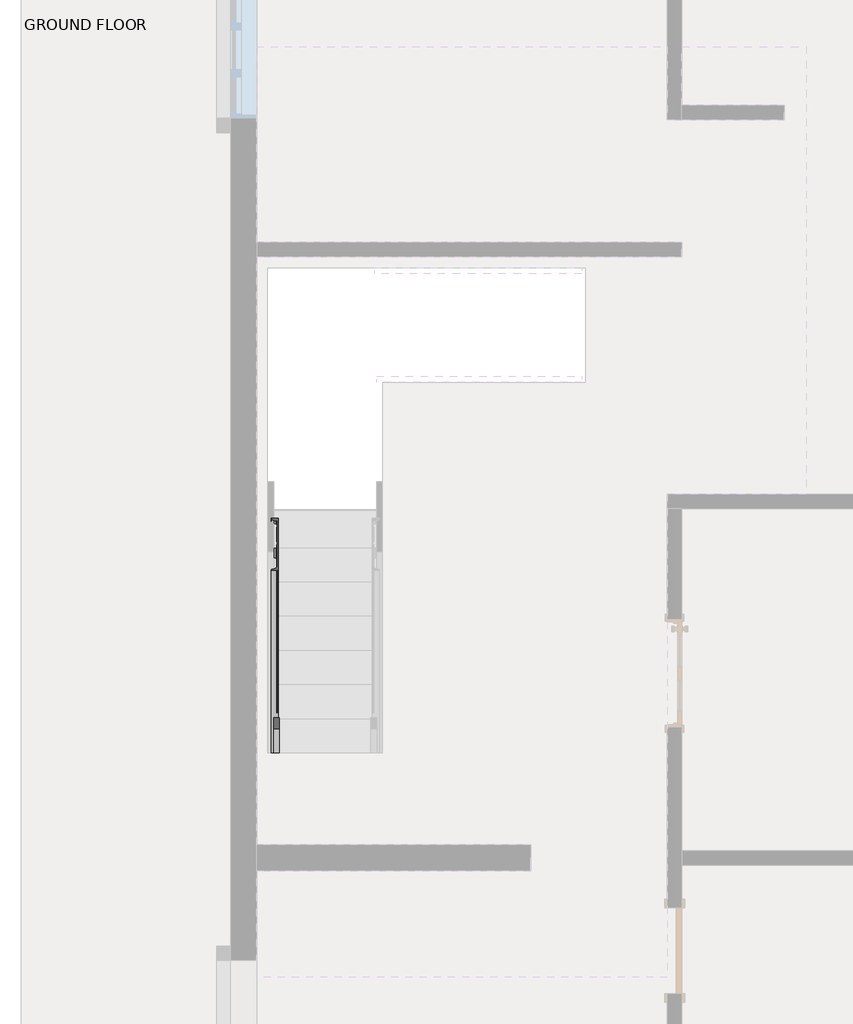
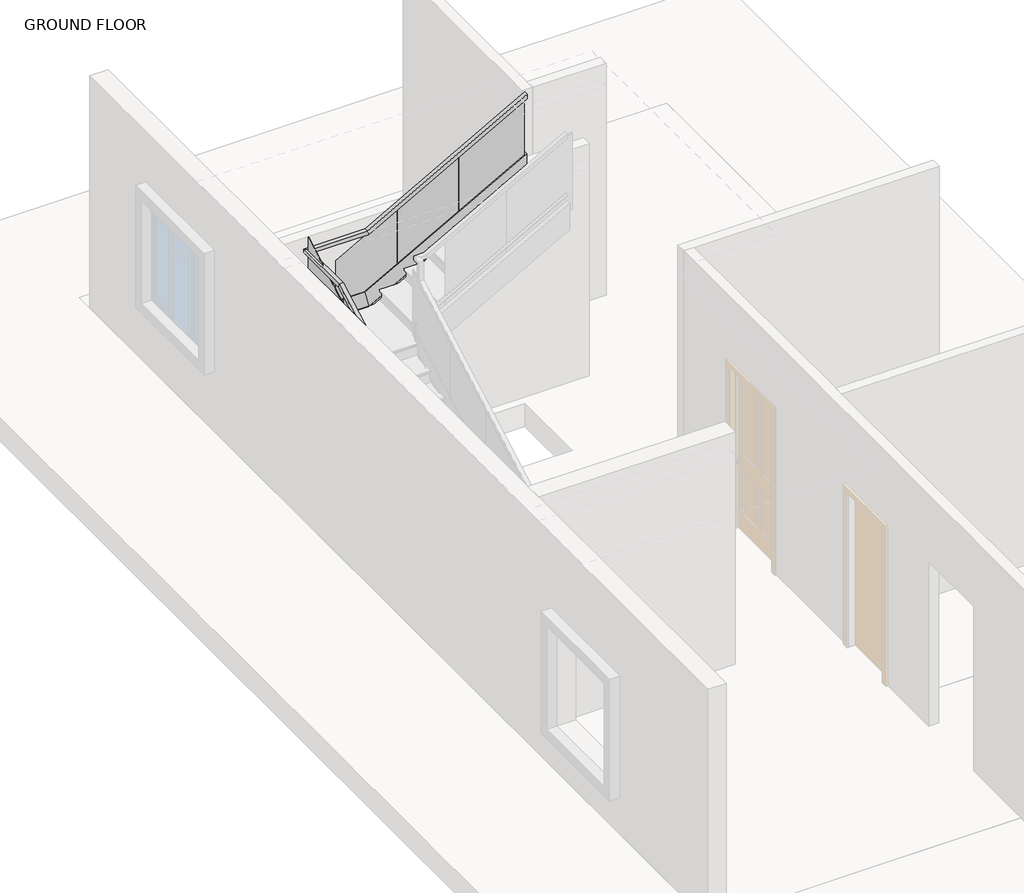
# One storey, part 3 of 4: 1 railing.
"""IFC4 building model written with IfcOpenShell, lengths in millimetres."""

from ifc_helpers import new_model, si_unit, frame, origin, place, context, project, spatial, polyline, circle_curve, ellipse_curve, outline, extrude, faceted_brep, element, save
from ifc_brep_helpers import plane_surface, cylinder_surface, revolved_surface, advanced_brep

model = new_model("IFC4")

# Units and contexts
model_context = context("Model", 3, world=origin())
ifc_project = project(units=[si_unit("LENGTHUNIT", "METRE", prefix="MILLI")], contexts=[model_context])

# Site, building, storey
site = spatial("IfcSite", under=ifc_project)
building = spatial("IfcBuilding", under=site)
storey = spatial("IfcBuildingStorey", under=building, Name="GROUND FLOOR", Elevation=304.8)

# Railing
placement = place(None, origin())
element("IfcRailing", 1, ObjectType="GLASS PANEL RAILING", at=placement, inside=storey, context=model_context, shape_type="SolidModel", body=[
    faceted_brep([(-9317.1482439, -642.5827462, 1388.5333333), (-9317.1482439, -642.5827462, 1330.420221), (-9266.3482439, -642.5827462, 1330.420221), (-9266.3482439, -642.5827462, 1388.5333333), (-9317.1482439, 2861.8235038, 3335.4256944), (-9317.1482439, 2874.9871061, 3284.6256944), (-9266.3482439, 2874.9871061, 3284.6256944), (-9266.3482439, 2861.8235038, 3335.4256944), (-9317.1482439, 3624.6172538, 3335.4256944), (-9317.1482439, 3624.6172538, 3284.6256944), (-9266.3482439, 3573.8172538, 3284.6256944), (-9266.3482439, 3573.8172538, 3335.4256944), (-8554.3544939, 3624.6172538, 3335.4256944), (-8541.1908917, 3624.6172538, 3284.6256944), (-8541.1908917, 3573.8172538, 3284.6256944), (-8554.3544939, 3573.8172538, 3335.4256944), (-6572.3607439, 3624.6172538, 4436.5333333), (-6572.3607439, 3573.8172538, 4436.5333333), (-6572.3607439, 3573.8172538, 4378.420221), (-6572.3607439, 3624.6172538, 4378.420221)], [[[0, 1, 2, 3]], [[1, 0, 4, 5]], [[2, 1, 5, 6]], [[3, 2, 6, 7]], [[0, 3, 7, 4]], [[5, 4, 8, 9]], [[6, 5, 9, 10]], [[7, 6, 10, 11]], [[4, 7, 11, 8]], [[9, 8, 12, 13]], [[10, 9, 13, 14]], [[11, 10, 14, 15]], [[8, 11, 15, 12]], [[16, 17, 18, 19]], [[13, 12, 16, 19]], [[14, 13, 19, 18]], [[15, 14, 18, 17]], [[12, 15, 17, 16]]]),
    advanced_brep(
    [(-9276.8638439, -642.5827462, 604.8878361), (-9340.1098439, -642.5827462, 604.8878361), (-9340.1098439, -642.5827462, 603.3095437), (-9335.7270347, -642.5827462, 597.391004), (-9312.1063439, -642.5827462, 592.8874784), (-9292.8684623, -642.5827462, 589.2195801), (-9284.1028439, -642.5827462, 577.3825008), (-9284.1028439, -642.5827462, 370.8841659), (-9292.8684623, -642.5827462, 359.0470866), (-9312.1063439, -642.5827462, 355.3791882), (-9335.7270347, -642.5827462, 350.8756626), (-9340.1098439, -642.5827462, 344.957123), (-9340.1098439, -642.5827462, 343.3788305), (-9276.8638439, -642.5827462, 343.3788305), (-9276.8638439, 2832.2053988, 2535.3256944), (-9340.1098439, 2832.2053988, 2535.3256944), (-9340.1098439, 2832.5629087, 2533.9460186), (-9335.7270347, 2833.903558, 2528.7722841), (-9312.1063439, 2834.9236827, 2524.8354944), (-9292.8684623, 2835.7545237, 2521.6291744), (-9284.1028439, 2838.4358222, 2511.2817054), (-9284.1028439, 2885.2111855, 2330.7696834), (-9292.8684623, 2887.892484, 2320.4222145), (-9312.1063439, 2888.723325, 2317.2158944), (-9335.7270347, 2889.7434497, 2313.2791048), (-9340.1098439, 2891.0840989, 2308.1053703), (-9340.1098439, 2891.4416089, 2306.7256944), (-9276.8638439, 2891.4416089, 2306.7256944), (-9276.8638439, 3584.3328538, 2535.3256944), (-9276.8638439, 3584.3328538, 2306.7256944), (-9340.1098439, 3584.3328538, 2306.7256944), (-9340.1098439, 3584.3328538, 2308.1053703), (-9335.7270347, 3584.3328538, 2313.2791048), (-9312.1063439, 3584.3328538, 2317.2158944), (-9292.8684623, 3584.3328538, 2320.4222145), (-9284.1028439, 3584.3328538, 2330.7696834), (-9284.1028439, 3584.3328538, 2511.2817054), (-9292.8684623, 3584.3328538, 2521.6291744), (-9312.1063439, 3584.3328538, 2524.8354944), (-9335.7270347, 3584.3328538, 2528.7722841), (-9340.1098439, 3584.3328538, 2533.9460186), (-9340.1098439, 3584.3328538, 2535.3256944)],
    [
        (0, 1),
        (1, 2),
        (2, 3, ellipse_curve(frame((-9334.8647439, -642.5827462, 603.3095437), z_axis=(0.0, -1.0, 0.0), x_axis=(0.0, 0.0, -1.0)), 6.0001789, 5.2451)),
        (3, 4),
        (4, 5),
        (5, 6, ellipse_curve(frame((-9294.5930439, -642.5827462, 577.3825008), z_axis=(0.0, 1.0, 0.0), x_axis=(0.0, 0.0, 1.0)), 12.0003577, 10.4902)),
        (6, 7),
        (7, 8, ellipse_curve(frame((-9294.5930439, -642.5827462, 370.8841659), z_axis=(0.0, 1.0, 0.0), x_axis=(0.0, 0.0, 1.0)), 12.0003577, 10.4902)),
        (8, 9),
        (9, 10),
        (10, 11, ellipse_curve(frame((-9334.8647439, -642.5827462, 344.957123), z_axis=(0.0, -1.0, 0.0), x_axis=(0.0, 0.0, -1.0)), 6.0001789, 5.2451)),
        (11, 12),
        (12, 13),
        (13, 0),
        (0, 14),
        (14, 15),
        (15, 1),
        (15, 16),
        (16, 2),
        (16, 17, ellipse_curve(frame((-9334.8647439, 2832.5629087, 2533.9460186), z_axis=(0.0, -0.9680282217274294, -0.25084130827922024), x_axis=(0.0, 0.25084130827922074, -0.9680282217274293)), 5.4183338, 5.2451)),
        (17, 3),
        (17, 18),
        (18, 4),
        (18, 19),
        (19, 5),
        (19, 20, ellipse_curve(frame((-9294.5930439, 2838.4358222, 2511.2817054), z_axis=(0.0, 0.9680282217274294, 0.25084130827922024), x_axis=(0.0, -0.25084130827922074, 0.9680282217274293)), 10.8366675, 10.4902)),
        (20, 6),
        (20, 21),
        (21, 7),
        (21, 22, ellipse_curve(frame((-9294.5930439, 2885.2111855, 2330.7696834), z_axis=(0.0, 0.9680282217274294, 0.25084130827922024), x_axis=(0.0, -0.25084130827922074, 0.9680282217274293)), 10.8366675, 10.4902)),
        (22, 8),
        (22, 23),
        (23, 9),
        (23, 24),
        (24, 10),
        (24, 25, ellipse_curve(frame((-9334.8647439, 2891.0840989, 2308.1053703), z_axis=(0.0, -0.9680282217274294, -0.25084130827922024), x_axis=(0.0, 0.25084130827922074, -0.9680282217274293)), 5.4183338, 5.2451)),
        (25, 11),
        (25, 26),
        (26, 12),
        (26, 27),
        (27, 13),
        (27, 14),
        (28, 29),
        (29, 30),
        (30, 31),
        (31, 32, circle_curve(frame((-9334.8647439, 3584.3328538, 2308.1053703), z_axis=(0.0, 1.0, 0.0), x_axis=(-1.0, 0.0, 0.0)), 5.2451)),
        (32, 33),
        (33, 34),
        (34, 35, circle_curve(frame((-9294.5930439, 3584.3328538, 2330.7696834), z_axis=(0.0, -1.0, 0.0), x_axis=(-1.0, 0.0, 0.0)), 10.4902)),
        (35, 36),
        (36, 37, circle_curve(frame((-9294.5930439, 3584.3328538, 2511.2817054), z_axis=(0.0, -1.0, 0.0), x_axis=(-1.0, 0.0, 0.0)), 10.4902)),
        (37, 38),
        (38, 39),
        (39, 40, circle_curve(frame((-9334.8647439, 3584.3328538, 2533.9460186), z_axis=(0.0, 1.0, 0.0), x_axis=(-1.0, 0.0, 0.0)), 5.2451)),
        (40, 41),
        (41, 28),
        (14, 28),
        (41, 15),
        (40, 16),
        (39, 17),
        (38, 18),
        (37, 19),
        (36, 20),
        (35, 21),
        (34, 22),
        (33, 23),
        (32, 24),
        (31, 25),
        (30, 26),
        (29, 27),
    ],
    [
        plane_surface(frame((-9291.7482439, -642.5827462, 474.1333333), z_axis=(0.0, -1.0, 0.0), x_axis=(0.0, 0.0, 1.0))),
        plane_surface(frame((-9276.8638439, -642.5827462, 604.8878361), z_axis=(0.0, -0.48564293117863094, 0.8741572761215385), x_axis=(0.0, 0.8741572761215385, 0.48564293117863094))),
        plane_surface(frame((-9340.1098439, -642.5827462, 604.8878361), z_axis=(-1.0, 0.0, 0.0), x_axis=(0.0, 0.8741572761215384, 0.4856429311786311))),
        cylinder_surface(frame((-9334.8647439, -697.4217034, 572.8434563), z_axis=(0.0, -0.8741572761215384, -0.48564293117863094), x_axis=(-1.0, 0.0, 0.0)), 5.2451),
        plane_surface(frame((-9335.7270347, -642.5827462, 597.391004), z_axis=(-0.16439930721687, 0.47903521057281384, -0.862263379031067), x_axis=(0.0, 0.8741572761215385, 0.48564293117863105))),
        plane_surface(frame((-9312.1063439, -642.5827462, 592.8874784), z_axis=(-0.16439930721687057, 0.4790352105728138, -0.8622633790310668), x_axis=(0.0, 0.8741572761215384, 0.48564293117863105))),
        revolved_surface(polyline([(-9305.0832439, 2840.8120297710066, 2512.6018208061087), (-9305.0832439, -647.677237685849, 574.5522277745283)]), (-9294.5930439, -686.4149399, 553.0312821), (0.0, 0.8741572761215384, 0.48564293117863094)),
        plane_surface(frame((-9284.1028439, -642.5827462, 577.3825008), z_axis=(-1.0, 0.0, 0.0), x_axis=(0.0, 0.8741572761215384, 0.485642931178631))),
        revolved_surface(polyline([(-9305.0832439, 2887.587393094591, 2332.0897987636554), (-9305.0832439, -647.6772376433962, 368.0538927981132)]), (-9294.5930439, -598.7505524, 395.2353846), (0.0, 0.8741572761215384, 0.48564293117863094)),
        plane_surface(frame((-9292.8684623, -642.5827462, 359.0470866), z_axis=(-0.16439930721687776, -0.4790352105728128, 0.862263379031066), x_axis=(0.0, 0.8741572761215384, 0.485642931178631))),
        plane_surface(frame((-9312.1063439, -642.5827462, 355.3791882), z_axis=(-0.1643993072168788, -0.4790352105728126, 0.8622633790310659), x_axis=(0.0, 0.8741572761215384, 0.48564293117863094))),
        cylinder_surface(frame((-9334.8647439, -587.7437889, 375.4232103), z_axis=(0.0, -0.8741572761215384, -0.48564293117863094), x_axis=(-1.0, 0.0, 0.0)), 5.2451),
        plane_surface(frame((-9340.1098439, -642.5827462, 344.957123), z_axis=(-1.0, 0.0, 0.0), x_axis=(0.0, 0.8741572761215384, 0.485642931178631))),
        plane_surface(frame((-9340.1098439, -642.5827462, 343.3788305), z_axis=(0.0, 0.48564293117863094, -0.8741572761215385), x_axis=(0.0, 0.8741572761215385, 0.48564293117863094))),
        plane_surface(frame((-9276.8638439, -642.5827462, 343.3788305), z_axis=(1.0000000000000002, 0.0, 0.0), x_axis=(0.0, 0.8741572761215385, 0.48564293117863094))),
        plane_surface(frame((-9291.7482439, 3584.3328538, 2421.0256944), z_axis=(0.0, 1.0, 0.0), x_axis=(0.0, 0.0, 1.0))),
        plane_surface(frame((-9276.8638439, 2832.2053988, 2535.3256944), z_axis=(0.0, 0.0, 1.0), x_axis=(0.0, 1.0, 0.0))),
        plane_surface(frame((-9340.1098439, 2832.2053988, 2535.3256944), z_axis=(-1.0, 0.0, 0.0), x_axis=(0.0, 1.0, 0.0))),
        cylinder_surface(frame((-9334.8647439, 2861.8235038, 2533.9460186), z_axis=(0.0, -1.0, 0.0), x_axis=(-1.0, 0.0, 0.0)), 5.2451),
        plane_surface(frame((-9335.7270347, 2833.903558, 2528.7722841), z_axis=(-0.16439930721687074, 0.0, -0.9863938705135049), x_axis=(0.0, 1.0, 0.0))),
        plane_surface(frame((-9312.1063439, 2834.9236827, 2524.8354944), z_axis=(-0.16439930721687138, 0.0, -0.9863938705135048), x_axis=(0.0, 1.0, 0.0))),
        revolved_surface(polyline([(-9305.0832439, 3584.3328538, 2511.2817054), (-9305.0832439, 2835.717538346913, 2511.2817054)]), (-9294.5930439, 2861.8235038, 2511.2817054), (0.0, 1.0, 0.0)),
        plane_surface(frame((-9284.1028439, 2838.4358222, 2511.2817054), z_axis=(-1.0, 0.0, 0.0), x_axis=(0.0, 1.0, 0.0))),
        revolved_surface(polyline([(-9305.0832439, 3584.3328538, 2330.7696834), (-9305.0832439, 2882.4929016469127, 2330.7696834)]), (-9294.5930439, 2861.8235038, 2330.7696834), (0.0, 1.0, 0.0)),
        plane_surface(frame((-9292.8684623, 2887.892484, 2320.4222145), z_axis=(-0.16439930721687698, 0.0, 0.9863938705135039), x_axis=(0.0, 1.0, 0.0))),
        plane_surface(frame((-9312.1063439, 2888.723325, 2317.2158944), z_axis=(-0.164399307216878, 0.0, 0.9863938705135037), x_axis=(0.0, 1.0, 0.0))),
        cylinder_surface(frame((-9334.8647439, 2861.8235038, 2308.1053703), z_axis=(0.0, -1.0, 0.0), x_axis=(-1.0, 0.0, 0.0)), 5.2451),
        plane_surface(frame((-9340.1098439, 2891.0840989, 2308.1053703), z_axis=(-1.0, 0.0, 0.0), x_axis=(0.0, 1.0, 0.0))),
        plane_surface(frame((-9340.1098439, 2891.4416089, 2306.7256944), z_axis=(0.0, 0.0, -1.0), x_axis=(0.0, 1.0, 0.0))),
        plane_surface(frame((-9276.8638439, 2891.4416089, 2306.7256944), z_axis=(1.0, 0.0, 0.0), x_axis=(0.0, 1.0, 0.0))),
    ],
    [
        (0, [[1, 2, 3, 4, 5, 6, 7, 8, 9, 10, 11, 12, 13, 14]]),
        (1, [[-1, 15, 16, 17]]),
        (2, [[-2, -17, 18, 19]]),
        (3, [[-3, -19, 20, 21]]),
        (4, [[-4, -21, 22, 23]]),
        (5, [[-5, -23, 24, 25]]),
        (6, [[-6, -25, 26, 27]]),
        (7, [[-7, -27, 28, 29]]),
        (8, [[-8, -29, 30, 31]]),
        (9, [[-9, -31, 32, 33]]),
        (10, [[-10, -33, 34, 35]]),
        (11, [[-11, -35, 36, 37]]),
        (12, [[-12, -37, 38, 39]]),
        (13, [[-13, -39, 40, 41]]),
        (14, [[-14, -41, 42, -15]]),
        (15, [[43, 44, 45, 46, 47, 48, 49, 50, 51, 52, 53, 54, 55, 56]]),
        (16, [[-16, 57, -56, 58]]),
        (17, [[-18, -58, -55, 59]]),
        (18, [[-20, -59, -54, 60]]),
        (19, [[-22, -60, -53, 61]]),
        (20, [[-24, -61, -52, 62]]),
        (21, [[-26, -62, -51, 63]]),
        (22, [[-28, -63, -50, 64]]),
        (23, [[-30, -64, -49, 65]]),
        (24, [[-32, -65, -48, 66]]),
        (25, [[-34, -66, -47, 67]]),
        (26, [[-36, -67, -46, 68]]),
        (27, [[-38, -68, -45, 69]]),
        (28, [[-40, -69, -44, 70]]),
        (29, [[-42, -70, -43, -57]]),
    ],
),
    advanced_brep(
    [(-9340.1098439, 3584.3328538, 2535.3256944), (-9340.1098439, 3647.5788538, 2535.3256944), (-9340.1098439, 3647.5788538, 2533.9460186), (-9340.1098439, 3643.1960447, 2528.7722841), (-9340.1098439, 3619.5753538, 2524.8354944), (-9340.1098439, 3600.3374722, 2521.6291744), (-9340.1098439, 3591.5718538, 2511.2817054), (-9340.1098439, 3591.5718538, 2330.7696834), (-9340.1098439, 3600.3374722, 2320.4222145), (-9340.1098439, 3619.5753538, 2317.2158944), (-9340.1098439, 3643.1960447, 2313.2791048), (-9340.1098439, 3647.5788538, 2308.1053703), (-9340.1098439, 3647.5788538, 2306.7256944), (-9340.1098439, 3584.3328538, 2306.7256944), (-8583.9725989, 3584.3328538, 2535.3256944), (-8583.9725989, 3647.5788538, 2535.3256944), (-8583.615089, 3647.5788538, 2533.9460186), (-8582.2744397, 3643.1960447, 2528.7722841), (-8581.2543151, 3619.5753538, 2524.8354944), (-8580.4234741, 3600.3374722, 2521.6291744), (-8577.7421756, 3591.5718538, 2511.2817054), (-8530.9668123, 3591.5718538, 2330.7696834), (-8528.2855137, 3600.3374722, 2320.4222145), (-8527.4546728, 3619.5753538, 2317.2158944), (-8526.4345481, 3643.1960447, 2313.2791048), (-8525.0938988, 3647.5788538, 2308.1053703), (-8524.7363889, 3647.5788538, 2306.7256944), (-8524.7363889, 3584.3328538, 2306.7256944), (-6572.3607439, 3584.3328538, 3652.8878361), (-6572.3607439, 3584.3328538, 3391.3788305), (-6572.3607439, 3647.5788538, 3391.3788305), (-6572.3607439, 3647.5788538, 3392.957123), (-6572.3607439, 3643.1960447, 3398.8756626), (-6572.3607439, 3619.5753538, 3403.3791882), (-6572.3607439, 3600.3374722, 3407.0470866), (-6572.3607439, 3591.5718538, 3418.8841659), (-6572.3607439, 3591.5718538, 3625.3825008), (-6572.3607439, 3600.3374722, 3637.2195801), (-6572.3607439, 3619.5753538, 3640.8874784), (-6572.3607439, 3643.1960447, 3645.391004), (-6572.3607439, 3647.5788538, 3651.3095437), (-6572.3607439, 3647.5788538, 3652.8878361)],
    [
        (0, 1),
        (1, 2),
        (2, 3, circle_curve(frame((-9340.1098439, 3642.3337538, 2533.9460186), z_axis=(-1.0, 0.0, 0.0), x_axis=(0.0, 1.0, 0.0)), 5.2451)),
        (3, 4),
        (4, 5),
        (5, 6, circle_curve(frame((-9340.1098439, 3602.0620538, 2511.2817054), z_axis=(1.0, 0.0, 0.0), x_axis=(0.0, 1.0, 0.0)), 10.4902)),
        (6, 7),
        (7, 8, circle_curve(frame((-9340.1098439, 3602.0620538, 2330.7696834), z_axis=(1.0, 0.0, 0.0), x_axis=(0.0, 1.0, 0.0)), 10.4902)),
        (8, 9),
        (9, 10),
        (10, 11, circle_curve(frame((-9340.1098439, 3642.3337538, 2308.1053703), z_axis=(-1.0, 0.0, 0.0), x_axis=(0.0, 1.0, 0.0)), 5.2451)),
        (11, 12),
        (12, 13),
        (13, 0),
        (0, 14),
        (14, 15),
        (15, 1),
        (15, 16),
        (16, 2),
        (16, 17, ellipse_curve(frame((-8583.615089, 3642.3337538, 2533.9460186), z_axis=(-0.9680282217274294, 0.0, -0.2508413082792203), x_axis=(-0.2508413082792198, 0.0, 0.9680282217274295)), 5.4183338, 5.2451)),
        (17, 3),
        (17, 18),
        (18, 4),
        (18, 19),
        (19, 5),
        (19, 20, ellipse_curve(frame((-8577.7421756, 3602.0620538, 2511.2817054), z_axis=(0.9680282217274294, 0.0, 0.2508413082792203), x_axis=(0.2508413082792198, 0.0, -0.9680282217274295)), 10.8366675, 10.4902)),
        (20, 6),
        (20, 21),
        (21, 7),
        (21, 22, ellipse_curve(frame((-8530.9668123, 3602.0620538, 2330.7696834), z_axis=(0.9680282217274294, 0.0, 0.2508413082792203), x_axis=(0.2508413082792198, 0.0, -0.9680282217274295)), 10.8366675, 10.4902)),
        (22, 8),
        (22, 23),
        (23, 9),
        (23, 24),
        (24, 10),
        (24, 25, ellipse_curve(frame((-8525.0938988, 3642.3337538, 2308.1053703), z_axis=(-0.9680282217274294, 0.0, -0.2508413082792203), x_axis=(-0.2508413082792198, 0.0, 0.9680282217274295)), 5.4183338, 5.2451)),
        (25, 11),
        (25, 26),
        (26, 12),
        (26, 27),
        (27, 13),
        (27, 14),
        (28, 29),
        (29, 30),
        (30, 31),
        (31, 32, ellipse_curve(frame((-6572.3607439, 3642.3337538, 3392.957123), z_axis=(1.0, 0.0, 0.0), x_axis=(0.0, 0.0, -1.0)), 6.0001789, 5.2451)),
        (32, 33),
        (33, 34),
        (34, 35, ellipse_curve(frame((-6572.3607439, 3602.0620538, 3418.8841659), z_axis=(-1.0, 0.0, 0.0), x_axis=(0.0, 0.0, 1.0)), 12.0003577, 10.4902)),
        (35, 36),
        (36, 37, ellipse_curve(frame((-6572.3607439, 3602.0620538, 3625.3825008), z_axis=(-1.0, 0.0, 0.0), x_axis=(0.0, 0.0, 1.0)), 12.0003577, 10.4902)),
        (37, 38),
        (38, 39),
        (39, 40, ellipse_curve(frame((-6572.3607439, 3642.3337538, 3651.3095437), z_axis=(1.0, 0.0, 0.0), x_axis=(0.0, 0.0, -1.0)), 6.0001789, 5.2451)),
        (40, 41),
        (41, 28),
        (14, 28),
        (41, 15),
        (40, 16),
        (39, 17),
        (38, 18),
        (37, 19),
        (36, 20),
        (35, 21),
        (34, 22),
        (33, 23),
        (32, 24),
        (31, 25),
        (30, 26),
        (29, 27),
    ],
    [
        plane_surface(frame((-9340.1098439, 3599.2172538, 2421.0256944), z_axis=(-1.0, 0.0, 0.0), x_axis=(0.0, 1.0, 0.0))),
        plane_surface(frame((-9340.1098439, 3584.3328538, 2535.3256944), z_axis=(0.0, 0.0, 1.0), x_axis=(1.0, 0.0, 0.0))),
        plane_surface(frame((-9340.1098439, 3647.5788538, 2535.3256944), z_axis=(0.0, 1.0, 0.0), x_axis=(1.0, 0.0, 0.0))),
        cylinder_surface(frame((-9340.1098439, 3642.3337538, 2533.9460186), z_axis=(-1.0, 0.0, 0.0), x_axis=(0.0, 1.0, 0.0)), 5.2451),
        plane_surface(frame((-9340.1098439, 3643.1960447, 2528.7722841), z_axis=(0.0, 0.16439930721687082, -0.9863938705135049), x_axis=(1.0, 0.0, 0.0))),
        plane_surface(frame((-9340.1098439, 3619.5753538, 2524.8354944), z_axis=(0.0, 0.16439930721687146, -0.9863938705135048), x_axis=(1.0, 0.0, 0.0))),
        revolved_surface(polyline([(-8575.023891746914, 3612.5522538, 2511.2817054), (-9340.1098439, 3612.5522538, 2511.2817054)]), (-9340.1098439, 3602.0620538, 2511.2817054), (1.0, 0.0, 0.0)),
        plane_surface(frame((-9340.1098439, 3591.5718538, 2511.2817054), z_axis=(0.0, 1.0, 0.0), x_axis=(1.0, 0.0, 0.0))),
        revolved_surface(polyline([(-8528.248528446913, 3612.5522538, 2330.7696834), (-9340.1098439, 3612.5522538, 2330.7696834)]), (-9340.1098439, 3602.0620538, 2330.7696834), (1.0, 0.0, 0.0)),
        plane_surface(frame((-9340.1098439, 3600.3374722, 2320.4222145), z_axis=(0.0, 0.1643993072168769, 0.9863938705135039), x_axis=(1.0, 0.0, 0.0))),
        plane_surface(frame((-9340.1098439, 3619.5753538, 2317.2158944), z_axis=(0.0, 0.16439930721687793, 0.9863938705135037), x_axis=(1.0, 0.0, 0.0))),
        cylinder_surface(frame((-9340.1098439, 3642.3337538, 2308.1053703), z_axis=(-1.0, 0.0, 0.0), x_axis=(0.0, 1.0, 0.0)), 5.2451),
        plane_surface(frame((-9340.1098439, 3647.5788538, 2308.1053703), z_axis=(0.0, 1.0, 0.0), x_axis=(1.0, 0.0, 0.0))),
        plane_surface(frame((-9340.1098439, 3647.5788538, 2306.7256944), z_axis=(0.0, 0.0, -1.0), x_axis=(1.0, 0.0, 0.0))),
        plane_surface(frame((-9340.1098439, 3584.3328538, 2306.7256944), z_axis=(0.0, -1.0, 0.0), x_axis=(1.0, 0.0, 0.0))),
        plane_surface(frame((-6572.3607439, 3599.2172538, 3522.1333333), z_axis=(1.0, 0.0, 0.0), x_axis=(0.0, 1.0, 0.0))),
        plane_surface(frame((-8583.9725989, 3584.3328538, 2535.3256944), z_axis=(-0.4856429311786311, 0.0, 0.8741572761215384), x_axis=(0.8741572761215384, 0.0, 0.4856429311786311))),
        plane_surface(frame((-8583.9725989, 3647.5788538, 2535.3256944), z_axis=(0.0, 1.0, 0.0), x_axis=(0.8741572761215384, 0.0, 0.4856429311786311))),
        cylinder_surface(frame((-8609.1934511, 3642.3337538, 2519.7358174), z_axis=(-0.8741572761215384, 0.0, -0.48564293117863105), x_axis=(0.0, 1.0, 0.0)), 5.2451),
        plane_surface(frame((-8582.2744397, 3643.1960447, 2528.7722841), z_axis=(0.47903521057281395, 0.1643993072168694, -0.862263379031067), x_axis=(0.8741572761215385, 0.0, 0.48564293117863094))),
        plane_surface(frame((-8581.2543151, 3619.5753538, 2524.8354944), z_axis=(0.47903521057281423, 0.16439930721687004, -0.8622633790310666), x_axis=(0.8741572761215383, 0.0, 0.4856429311786313))),
        revolved_surface(polyline([(-6567.2662524518855, 3612.5522538, 3628.212773893393), (-8580.11838324176, 3612.5522538, 2509.9615901212446)]), (-8598.1866877, 3602.0620538, 2499.9236432), (0.8741572761215384, 0.0, 0.48564293117863105)),
        plane_surface(frame((-8577.7421756, 3591.5718538, 2511.2817054), z_axis=(0.0, 1.0000000000000002, 0.0), x_axis=(0.8741572761215385, 0.0, 0.48564293117863094))),
        revolved_surface(polyline([(-6567.266252409432, 3612.5522538, 3421.714438916979), (-8533.343019918173, 3612.5522538, 2329.449568078793)]), (-8510.5223002, 3602.0620538, 2342.1277457), (0.8741572761215384, 0.0, 0.48564293117863105)),
        plane_surface(frame((-8528.2855137, 3600.3374722, 2320.4222145), z_axis=(-0.4790352105728125, 0.16439930721687834, 0.8622633790310661), x_axis=(0.8741572761215384, 0.0, 0.48564293117863094))),
        plane_surface(frame((-8527.4546728, 3619.5753538, 2317.2158944), z_axis=(-0.4790352105728125, 0.16439930721687937, 0.8622633790310658), x_axis=(0.8741572761215384, 0.0, 0.4856429311786311))),
        cylinder_surface(frame((-8499.5155367, 3642.3337538, 2322.3155715), z_axis=(-0.8741572761215384, 0.0, -0.48564293117863105), x_axis=(0.0, 1.0, 0.0)), 5.2451),
        plane_surface(frame((-8525.0938988, 3647.5788538, 2308.1053703), z_axis=(0.0, 1.0, 0.0), x_axis=(0.8741572761215384, 0.0, 0.4856429311786311))),
        plane_surface(frame((-8524.7363889, 3647.5788538, 2306.7256944), z_axis=(0.4856429311786312, 0.0, -0.8741572761215383), x_axis=(0.8741572761215383, 0.0, 0.4856429311786312))),
        plane_surface(frame((-8524.7363889, 3584.3328538, 2306.7256944), z_axis=(0.0, -1.0000000000000002, 0.0), x_axis=(0.8741572761215384, 0.0, 0.48564293117863117))),
    ],
    [
        (0, [[1, 2, 3, 4, 5, 6, 7, 8, 9, 10, 11, 12, 13, 14]]),
        (1, [[-1, 15, 16, 17]]),
        (2, [[-2, -17, 18, 19]]),
        (3, [[-3, -19, 20, 21]]),
        (4, [[-4, -21, 22, 23]]),
        (5, [[-5, -23, 24, 25]]),
        (6, [[-6, -25, 26, 27]]),
        (7, [[-7, -27, 28, 29]]),
        (8, [[-8, -29, 30, 31]]),
        (9, [[-9, -31, 32, 33]]),
        (10, [[-10, -33, 34, 35]]),
        (11, [[-11, -35, 36, 37]]),
        (12, [[-12, -37, 38, 39]]),
        (13, [[-13, -39, 40, 41]]),
        (14, [[-14, -41, 42, -15]]),
        (15, [[43, 44, 45, 46, 47, 48, 49, 50, 51, 52, 53, 54, 55, 56]]),
        (16, [[-16, 57, -56, 58]]),
        (17, [[-18, -58, -55, 59]]),
        (18, [[-20, -59, -54, 60]]),
        (19, [[-22, -60, -53, 61]]),
        (20, [[-24, -61, -52, 62]]),
        (21, [[-26, -62, -51, 63]]),
        (22, [[-28, -63, -50, 64]]),
        (23, [[-30, -64, -49, 65]]),
        (24, [[-32, -65, -48, 66]]),
        (25, [[-34, -66, -47, 67]]),
        (26, [[-36, -67, -46, 68]]),
        (27, [[-38, -68, -45, 69]]),
        (28, [[-40, -69, -44, 70]]),
        (29, [[-42, -70, -43, -57]]),
    ],
),
    advanced_brep(
    [(-9276.8638439, -642.5827462, 604.8878361), (-9340.1098439, -642.5827462, 604.8878361), (-9340.1098439, -642.5827462, 603.3095437), (-9335.7270347, -642.5827462, 597.391004), (-9312.1063439, -642.5827462, 592.8874784), (-9292.8684623, -642.5827462, 589.2195801), (-9284.1028439, -642.5827462, 577.3825008), (-9284.1028439, -642.5827462, 370.8841659), (-9292.8684623, -642.5827462, 359.0470866), (-9312.1063439, -642.5827462, 355.3791882), (-9335.7270347, -642.5827462, 350.8756626), (-9340.1098439, -642.5827462, 344.957123), (-9340.1098439, -642.5827462, 343.3788305), (-9276.8638439, -642.5827462, 343.3788305), (-9276.8638439, 2832.2053988, 2535.3256944), (-9340.1098439, 2832.2053988, 2535.3256944), (-9340.1098439, 2832.5629087, 2533.9460186), (-9335.7270347, 2833.903558, 2528.7722841), (-9312.1063439, 2834.9236827, 2524.8354944), (-9292.8684623, 2835.7545237, 2521.6291744), (-9284.1028439, 2838.4358222, 2511.2817054), (-9284.1028439, 2885.2111855, 2330.7696834), (-9292.8684623, 2887.892484, 2320.4222145), (-9312.1063439, 2888.723325, 2317.2158944), (-9335.7270347, 2889.7434497, 2313.2791048), (-9340.1098439, 2891.0840989, 2308.1053703), (-9340.1098439, 2891.4416089, 2306.7256944), (-9276.8638439, 2891.4416089, 2306.7256944), (-9276.8638439, 3584.3328538, 2535.3256944), (-9276.8638439, 3584.3328538, 2306.7256944), (-9340.1098439, 3584.3328538, 2306.7256944), (-9340.1098439, 3584.3328538, 2308.1053703), (-9335.7270347, 3584.3328538, 2313.2791048), (-9312.1063439, 3584.3328538, 2317.2158944), (-9292.8684623, 3584.3328538, 2320.4222145), (-9284.1028439, 3584.3328538, 2330.7696834), (-9284.1028439, 3584.3328538, 2511.2817054), (-9292.8684623, 3584.3328538, 2521.6291744), (-9312.1063439, 3584.3328538, 2524.8354944), (-9335.7270347, 3584.3328538, 2528.7722841), (-9340.1098439, 3584.3328538, 2533.9460186), (-9340.1098439, 3584.3328538, 2535.3256944)],
    [
        (0, 1),
        (1, 2),
        (2, 3, ellipse_curve(frame((-9334.8647439, -642.5827462, 603.3095437), z_axis=(0.0, -1.0, 0.0), x_axis=(0.0, 0.0, -1.0)), 6.0001789, 5.2451)),
        (3, 4),
        (4, 5),
        (5, 6, ellipse_curve(frame((-9294.5930439, -642.5827462, 577.3825008), z_axis=(0.0, 1.0, 0.0), x_axis=(0.0, 0.0, 1.0)), 12.0003577, 10.4902)),
        (6, 7),
        (7, 8, ellipse_curve(frame((-9294.5930439, -642.5827462, 370.8841659), z_axis=(0.0, 1.0, 0.0), x_axis=(0.0, 0.0, 1.0)), 12.0003577, 10.4902)),
        (8, 9),
        (9, 10),
        (10, 11, ellipse_curve(frame((-9334.8647439, -642.5827462, 344.957123), z_axis=(0.0, -1.0, 0.0), x_axis=(0.0, 0.0, -1.0)), 6.0001789, 5.2451)),
        (11, 12),
        (12, 13),
        (13, 0),
        (0, 14),
        (14, 15),
        (15, 1),
        (15, 16),
        (16, 2),
        (16, 17, ellipse_curve(frame((-9334.8647439, 2832.5629087, 2533.9460186), z_axis=(0.0, -0.9680282217274294, -0.25084130827922024), x_axis=(0.0, 0.25084130827922074, -0.9680282217274293)), 5.4183338, 5.2451)),
        (17, 3),
        (17, 18),
        (18, 4),
        (18, 19),
        (19, 5),
        (19, 20, ellipse_curve(frame((-9294.5930439, 2838.4358222, 2511.2817054), z_axis=(0.0, 0.9680282217274294, 0.25084130827922024), x_axis=(0.0, -0.25084130827922074, 0.9680282217274293)), 10.8366675, 10.4902)),
        (20, 6),
        (20, 21),
        (21, 7),
        (21, 22, ellipse_curve(frame((-9294.5930439, 2885.2111855, 2330.7696834), z_axis=(0.0, 0.9680282217274294, 0.25084130827922024), x_axis=(0.0, -0.25084130827922074, 0.9680282217274293)), 10.8366675, 10.4902)),
        (22, 8),
        (22, 23),
        (23, 9),
        (23, 24),
        (24, 10),
        (24, 25, ellipse_curve(frame((-9334.8647439, 2891.0840989, 2308.1053703), z_axis=(0.0, -0.9680282217274294, -0.25084130827922024), x_axis=(0.0, 0.25084130827922074, -0.9680282217274293)), 5.4183338, 5.2451)),
        (25, 11),
        (25, 26),
        (26, 12),
        (26, 27),
        (27, 13),
        (27, 14),
        (28, 29),
        (29, 30),
        (30, 31),
        (31, 32, circle_curve(frame((-9334.8647439, 3584.3328538, 2308.1053703), z_axis=(0.0, 1.0, 0.0), x_axis=(-1.0, 0.0, 0.0)), 5.2451)),
        (32, 33),
        (33, 34),
        (34, 35, circle_curve(frame((-9294.5930439, 3584.3328538, 2330.7696834), z_axis=(0.0, -1.0, 0.0), x_axis=(-1.0, 0.0, 0.0)), 10.4902)),
        (35, 36),
        (36, 37, circle_curve(frame((-9294.5930439, 3584.3328538, 2511.2817054), z_axis=(0.0, -1.0, 0.0), x_axis=(-1.0, 0.0, 0.0)), 10.4902)),
        (37, 38),
        (38, 39),
        (39, 40, circle_curve(frame((-9334.8647439, 3584.3328538, 2533.9460186), z_axis=(0.0, 1.0, 0.0), x_axis=(-1.0, 0.0, 0.0)), 5.2451)),
        (40, 41),
        (41, 28),
        (14, 28),
        (41, 15),
        (40, 16),
        (39, 17),
        (38, 18),
        (37, 19),
        (36, 20),
        (35, 21),
        (34, 22),
        (33, 23),
        (32, 24),
        (31, 25),
        (30, 26),
        (29, 27),
    ],
    [
        plane_surface(frame((-9291.7482439, -642.5827462, 474.1333333), z_axis=(0.0, -1.0, 0.0), x_axis=(0.0, 0.0, 1.0))),
        plane_surface(frame((-9276.8638439, -642.5827462, 604.8878361), z_axis=(0.0, -0.48564293117863094, 0.8741572761215385), x_axis=(0.0, 0.8741572761215385, 0.48564293117863094))),
        plane_surface(frame((-9340.1098439, -642.5827462, 604.8878361), z_axis=(-1.0, 0.0, 0.0), x_axis=(0.0, 0.8741572761215384, 0.4856429311786311))),
        cylinder_surface(frame((-9334.8647439, -697.4217034, 572.8434563), z_axis=(0.0, -0.8741572761215384, -0.48564293117863094), x_axis=(-1.0, 0.0, 0.0)), 5.2451),
        plane_surface(frame((-9335.7270347, -642.5827462, 597.391004), z_axis=(-0.16439930721687, 0.47903521057281384, -0.862263379031067), x_axis=(0.0, 0.8741572761215385, 0.48564293117863105))),
        plane_surface(frame((-9312.1063439, -642.5827462, 592.8874784), z_axis=(-0.16439930721687057, 0.4790352105728138, -0.8622633790310668), x_axis=(0.0, 0.8741572761215384, 0.48564293117863105))),
        revolved_surface(polyline([(-9305.0832439, 2840.8120297710066, 2512.6018208061087), (-9305.0832439, -647.677237685849, 574.5522277745283)]), (-9294.5930439, -686.4149399, 553.0312821), (0.0, 0.8741572761215384, 0.48564293117863094)),
        plane_surface(frame((-9284.1028439, -642.5827462, 577.3825008), z_axis=(-1.0, 0.0, 0.0), x_axis=(0.0, 0.8741572761215384, 0.485642931178631))),
        revolved_surface(polyline([(-9305.0832439, 2887.587393094591, 2332.0897987636554), (-9305.0832439, -647.6772376433962, 368.0538927981132)]), (-9294.5930439, -598.7505524, 395.2353846), (0.0, 0.8741572761215384, 0.48564293117863094)),
        plane_surface(frame((-9292.8684623, -642.5827462, 359.0470866), z_axis=(-0.16439930721687776, -0.4790352105728128, 0.862263379031066), x_axis=(0.0, 0.8741572761215384, 0.485642931178631))),
        plane_surface(frame((-9312.1063439, -642.5827462, 355.3791882), z_axis=(-0.1643993072168788, -0.4790352105728126, 0.8622633790310659), x_axis=(0.0, 0.8741572761215384, 0.48564293117863094))),
        cylinder_surface(frame((-9334.8647439, -587.7437889, 375.4232103), z_axis=(0.0, -0.8741572761215384, -0.48564293117863094), x_axis=(-1.0, 0.0, 0.0)), 5.2451),
        plane_surface(frame((-9340.1098439, -642.5827462, 344.957123), z_axis=(-1.0, 0.0, 0.0), x_axis=(0.0, 0.8741572761215384, 0.485642931178631))),
        plane_surface(frame((-9340.1098439, -642.5827462, 343.3788305), z_axis=(0.0, 0.48564293117863094, -0.8741572761215385), x_axis=(0.0, 0.8741572761215385, 0.48564293117863094))),
        plane_surface(frame((-9276.8638439, -642.5827462, 343.3788305), z_axis=(1.0000000000000002, 0.0, 0.0), x_axis=(0.0, 0.8741572761215385, 0.48564293117863094))),
        plane_surface(frame((-9291.7482439, 3584.3328538, 2421.0256944), z_axis=(0.0, 1.0, 0.0), x_axis=(0.0, 0.0, 1.0))),
        plane_surface(frame((-9276.8638439, 2832.2053988, 2535.3256944), z_axis=(0.0, 0.0, 1.0), x_axis=(0.0, 1.0, 0.0))),
        plane_surface(frame((-9340.1098439, 2832.2053988, 2535.3256944), z_axis=(-1.0, 0.0, 0.0), x_axis=(0.0, 1.0, 0.0))),
        cylinder_surface(frame((-9334.8647439, 2861.8235038, 2533.9460186), z_axis=(0.0, -1.0, 0.0), x_axis=(-1.0, 0.0, 0.0)), 5.2451),
        plane_surface(frame((-9335.7270347, 2833.903558, 2528.7722841), z_axis=(-0.16439930721687074, 0.0, -0.9863938705135049), x_axis=(0.0, 1.0, 0.0))),
        plane_surface(frame((-9312.1063439, 2834.9236827, 2524.8354944), z_axis=(-0.16439930721687138, 0.0, -0.9863938705135048), x_axis=(0.0, 1.0, 0.0))),
        revolved_surface(polyline([(-9305.0832439, 3584.3328538, 2511.2817054), (-9305.0832439, 2835.717538346913, 2511.2817054)]), (-9294.5930439, 2861.8235038, 2511.2817054), (0.0, 1.0, 0.0)),
        plane_surface(frame((-9284.1028439, 2838.4358222, 2511.2817054), z_axis=(-1.0, 0.0, 0.0), x_axis=(0.0, 1.0, 0.0))),
        revolved_surface(polyline([(-9305.0832439, 3584.3328538, 2330.7696834), (-9305.0832439, 2882.4929016469127, 2330.7696834)]), (-9294.5930439, 2861.8235038, 2330.7696834), (0.0, 1.0, 0.0)),
        plane_surface(frame((-9292.8684623, 2887.892484, 2320.4222145), z_axis=(-0.16439930721687698, 0.0, 0.9863938705135039), x_axis=(0.0, 1.0, 0.0))),
        plane_surface(frame((-9312.1063439, 2888.723325, 2317.2158944), z_axis=(-0.164399307216878, 0.0, 0.9863938705135037), x_axis=(0.0, 1.0, 0.0))),
        cylinder_surface(frame((-9334.8647439, 2861.8235038, 2308.1053703), z_axis=(0.0, -1.0, 0.0), x_axis=(-1.0, 0.0, 0.0)), 5.2451),
        plane_surface(frame((-9340.1098439, 2891.0840989, 2308.1053703), z_axis=(-1.0, 0.0, 0.0), x_axis=(0.0, 1.0, 0.0))),
        plane_surface(frame((-9340.1098439, 2891.4416089, 2306.7256944), z_axis=(0.0, 0.0, -1.0), x_axis=(0.0, 1.0, 0.0))),
        plane_surface(frame((-9276.8638439, 2891.4416089, 2306.7256944), z_axis=(1.0, 0.0, 0.0), x_axis=(0.0, 1.0, 0.0))),
    ],
    [
        (0, [[1, 2, 3, 4, 5, 6, 7, 8, 9, 10, 11, 12, 13, 14]]),
        (1, [[-1, 15, 16, 17]]),
        (2, [[-2, -17, 18, 19]]),
        (3, [[-3, -19, 20, 21]]),
        (4, [[-4, -21, 22, 23]]),
        (5, [[-5, -23, 24, 25]]),
        (6, [[-6, -25, 26, 27]]),
        (7, [[-7, -27, 28, 29]]),
        (8, [[-8, -29, 30, 31]]),
        (9, [[-9, -31, 32, 33]]),
        (10, [[-10, -33, 34, 35]]),
        (11, [[-11, -35, 36, 37]]),
        (12, [[-12, -37, 38, 39]]),
        (13, [[-13, -39, 40, 41]]),
        (14, [[-14, -41, 42, -15]]),
        (15, [[43, 44, 45, 46, 47, 48, 49, 50, 51, 52, 53, 54, 55, 56]]),
        (16, [[-16, 57, -56, 58]]),
        (17, [[-18, -58, -55, 59]]),
        (18, [[-20, -59, -54, 60]]),
        (19, [[-22, -60, -53, 61]]),
        (20, [[-24, -61, -52, 62]]),
        (21, [[-26, -62, -51, 63]]),
        (22, [[-28, -63, -50, 64]]),
        (23, [[-30, -64, -49, 65]]),
        (24, [[-32, -65, -48, 66]]),
        (25, [[-34, -66, -47, 67]]),
        (26, [[-36, -67, -46, 68]]),
        (27, [[-38, -68, -45, 69]]),
        (28, [[-40, -69, -44, 70]]),
        (29, [[-42, -70, -43, -57]]),
    ],
),
    advanced_brep(
    [(-9340.1098439, 3584.3328538, 2535.3256944), (-9340.1098439, 3647.5788538, 2535.3256944), (-9340.1098439, 3647.5788538, 2533.9460186), (-9340.1098439, 3643.1960447, 2528.7722841), (-9340.1098439, 3619.5753538, 2524.8354944), (-9340.1098439, 3600.3374722, 2521.6291744), (-9340.1098439, 3591.5718538, 2511.2817054), (-9340.1098439, 3591.5718538, 2330.7696834), (-9340.1098439, 3600.3374722, 2320.4222145), (-9340.1098439, 3619.5753538, 2317.2158944), (-9340.1098439, 3643.1960447, 2313.2791048), (-9340.1098439, 3647.5788538, 2308.1053703), (-9340.1098439, 3647.5788538, 2306.7256944), (-9340.1098439, 3584.3328538, 2306.7256944), (-8583.9725989, 3584.3328538, 2535.3256944), (-8583.9725989, 3647.5788538, 2535.3256944), (-8583.615089, 3647.5788538, 2533.9460186), (-8582.2744397, 3643.1960447, 2528.7722841), (-8581.2543151, 3619.5753538, 2524.8354944), (-8580.4234741, 3600.3374722, 2521.6291744), (-8577.7421756, 3591.5718538, 2511.2817054), (-8530.9668123, 3591.5718538, 2330.7696834), (-8528.2855137, 3600.3374722, 2320.4222145), (-8527.4546728, 3619.5753538, 2317.2158944), (-8526.4345481, 3643.1960447, 2313.2791048), (-8525.0938988, 3647.5788538, 2308.1053703), (-8524.7363889, 3647.5788538, 2306.7256944), (-8524.7363889, 3584.3328538, 2306.7256944), (-6572.3607439, 3584.3328538, 3652.8878361), (-6572.3607439, 3584.3328538, 3391.3788305), (-6572.3607439, 3647.5788538, 3391.3788305), (-6572.3607439, 3647.5788538, 3392.957123), (-6572.3607439, 3643.1960447, 3398.8756626), (-6572.3607439, 3619.5753538, 3403.3791882), (-6572.3607439, 3600.3374722, 3407.0470866), (-6572.3607439, 3591.5718538, 3418.8841659), (-6572.3607439, 3591.5718538, 3625.3825008), (-6572.3607439, 3600.3374722, 3637.2195801), (-6572.3607439, 3619.5753538, 3640.8874784), (-6572.3607439, 3643.1960447, 3645.391004), (-6572.3607439, 3647.5788538, 3651.3095437), (-6572.3607439, 3647.5788538, 3652.8878361)],
    [
        (0, 1),
        (1, 2),
        (2, 3, circle_curve(frame((-9340.1098439, 3642.3337538, 2533.9460186), z_axis=(-1.0, 0.0, 0.0), x_axis=(0.0, 1.0, 0.0)), 5.2451)),
        (3, 4),
        (4, 5),
        (5, 6, circle_curve(frame((-9340.1098439, 3602.0620538, 2511.2817054), z_axis=(1.0, 0.0, 0.0), x_axis=(0.0, 1.0, 0.0)), 10.4902)),
        (6, 7),
        (7, 8, circle_curve(frame((-9340.1098439, 3602.0620538, 2330.7696834), z_axis=(1.0, 0.0, 0.0), x_axis=(0.0, 1.0, 0.0)), 10.4902)),
        (8, 9),
        (9, 10),
        (10, 11, circle_curve(frame((-9340.1098439, 3642.3337538, 2308.1053703), z_axis=(-1.0, 0.0, 0.0), x_axis=(0.0, 1.0, 0.0)), 5.2451)),
        (11, 12),
        (12, 13),
        (13, 0),
        (0, 14),
        (14, 15),
        (15, 1),
        (15, 16),
        (16, 2),
        (16, 17, ellipse_curve(frame((-8583.615089, 3642.3337538, 2533.9460186), z_axis=(-0.9680282217274294, 0.0, -0.2508413082792203), x_axis=(-0.2508413082792198, 0.0, 0.9680282217274295)), 5.4183338, 5.2451)),
        (17, 3),
        (17, 18),
        (18, 4),
        (18, 19),
        (19, 5),
        (19, 20, ellipse_curve(frame((-8577.7421756, 3602.0620538, 2511.2817054), z_axis=(0.9680282217274294, 0.0, 0.2508413082792203), x_axis=(0.2508413082792198, 0.0, -0.9680282217274295)), 10.8366675, 10.4902)),
        (20, 6),
        (20, 21),
        (21, 7),
        (21, 22, ellipse_curve(frame((-8530.9668123, 3602.0620538, 2330.7696834), z_axis=(0.9680282217274294, 0.0, 0.2508413082792203), x_axis=(0.2508413082792198, 0.0, -0.9680282217274295)), 10.8366675, 10.4902)),
        (22, 8),
        (22, 23),
        (23, 9),
        (23, 24),
        (24, 10),
        (24, 25, ellipse_curve(frame((-8525.0938988, 3642.3337538, 2308.1053703), z_axis=(-0.9680282217274294, 0.0, -0.2508413082792203), x_axis=(-0.2508413082792198, 0.0, 0.9680282217274295)), 5.4183338, 5.2451)),
        (25, 11),
        (25, 26),
        (26, 12),
        (26, 27),
        (27, 13),
        (27, 14),
        (28, 29),
        (29, 30),
        (30, 31),
        (31, 32, ellipse_curve(frame((-6572.3607439, 3642.3337538, 3392.957123), z_axis=(1.0, 0.0, 0.0), x_axis=(0.0, 0.0, -1.0)), 6.0001789, 5.2451)),
        (32, 33),
        (33, 34),
        (34, 35, ellipse_curve(frame((-6572.3607439, 3602.0620538, 3418.8841659), z_axis=(-1.0, 0.0, 0.0), x_axis=(0.0, 0.0, 1.0)), 12.0003577, 10.4902)),
        (35, 36),
        (36, 37, ellipse_curve(frame((-6572.3607439, 3602.0620538, 3625.3825008), z_axis=(-1.0, 0.0, 0.0), x_axis=(0.0, 0.0, 1.0)), 12.0003577, 10.4902)),
        (37, 38),
        (38, 39),
        (39, 40, ellipse_curve(frame((-6572.3607439, 3642.3337538, 3651.3095437), z_axis=(1.0, 0.0, 0.0), x_axis=(0.0, 0.0, -1.0)), 6.0001789, 5.2451)),
        (40, 41),
        (41, 28),
        (14, 28),
        (41, 15),
        (40, 16),
        (39, 17),
        (38, 18),
        (37, 19),
        (36, 20),
        (35, 21),
        (34, 22),
        (33, 23),
        (32, 24),
        (31, 25),
        (30, 26),
        (29, 27),
    ],
    [
        plane_surface(frame((-9340.1098439, 3599.2172538, 2421.0256944), z_axis=(-1.0, 0.0, 0.0), x_axis=(0.0, 1.0, 0.0))),
        plane_surface(frame((-9340.1098439, 3584.3328538, 2535.3256944), z_axis=(0.0, 0.0, 1.0), x_axis=(1.0, 0.0, 0.0))),
        plane_surface(frame((-9340.1098439, 3647.5788538, 2535.3256944), z_axis=(0.0, 1.0, 0.0), x_axis=(1.0, 0.0, 0.0))),
        cylinder_surface(frame((-9340.1098439, 3642.3337538, 2533.9460186), z_axis=(-1.0, 0.0, 0.0), x_axis=(0.0, 1.0, 0.0)), 5.2451),
        plane_surface(frame((-9340.1098439, 3643.1960447, 2528.7722841), z_axis=(0.0, 0.16439930721687082, -0.9863938705135049), x_axis=(1.0, 0.0, 0.0))),
        plane_surface(frame((-9340.1098439, 3619.5753538, 2524.8354944), z_axis=(0.0, 0.16439930721687146, -0.9863938705135048), x_axis=(1.0, 0.0, 0.0))),
        revolved_surface(polyline([(-8575.023891746914, 3612.5522538, 2511.2817054), (-9340.1098439, 3612.5522538, 2511.2817054)]), (-9340.1098439, 3602.0620538, 2511.2817054), (1.0, 0.0, 0.0)),
        plane_surface(frame((-9340.1098439, 3591.5718538, 2511.2817054), z_axis=(0.0, 1.0, 0.0), x_axis=(1.0, 0.0, 0.0))),
        revolved_surface(polyline([(-8528.248528446913, 3612.5522538, 2330.7696834), (-9340.1098439, 3612.5522538, 2330.7696834)]), (-9340.1098439, 3602.0620538, 2330.7696834), (1.0, 0.0, 0.0)),
        plane_surface(frame((-9340.1098439, 3600.3374722, 2320.4222145), z_axis=(0.0, 0.1643993072168769, 0.9863938705135039), x_axis=(1.0, 0.0, 0.0))),
        plane_surface(frame((-9340.1098439, 3619.5753538, 2317.2158944), z_axis=(0.0, 0.16439930721687793, 0.9863938705135037), x_axis=(1.0, 0.0, 0.0))),
        cylinder_surface(frame((-9340.1098439, 3642.3337538, 2308.1053703), z_axis=(-1.0, 0.0, 0.0), x_axis=(0.0, 1.0, 0.0)), 5.2451),
        plane_surface(frame((-9340.1098439, 3647.5788538, 2308.1053703), z_axis=(0.0, 1.0, 0.0), x_axis=(1.0, 0.0, 0.0))),
        plane_surface(frame((-9340.1098439, 3647.5788538, 2306.7256944), z_axis=(0.0, 0.0, -1.0), x_axis=(1.0, 0.0, 0.0))),
        plane_surface(frame((-9340.1098439, 3584.3328538, 2306.7256944), z_axis=(0.0, -1.0, 0.0), x_axis=(1.0, 0.0, 0.0))),
        plane_surface(frame((-6572.3607439, 3599.2172538, 3522.1333333), z_axis=(1.0, 0.0, 0.0), x_axis=(0.0, 1.0, 0.0))),
        plane_surface(frame((-8583.9725989, 3584.3328538, 2535.3256944), z_axis=(-0.4856429311786311, 0.0, 0.8741572761215384), x_axis=(0.8741572761215384, 0.0, 0.4856429311786311))),
        plane_surface(frame((-8583.9725989, 3647.5788538, 2535.3256944), z_axis=(0.0, 1.0, 0.0), x_axis=(0.8741572761215384, 0.0, 0.4856429311786311))),
        cylinder_surface(frame((-8609.1934511, 3642.3337538, 2519.7358174), z_axis=(-0.8741572761215384, 0.0, -0.48564293117863105), x_axis=(0.0, 1.0, 0.0)), 5.2451),
        plane_surface(frame((-8582.2744397, 3643.1960447, 2528.7722841), z_axis=(0.47903521057281395, 0.1643993072168694, -0.862263379031067), x_axis=(0.8741572761215385, 0.0, 0.48564293117863094))),
        plane_surface(frame((-8581.2543151, 3619.5753538, 2524.8354944), z_axis=(0.47903521057281423, 0.16439930721687004, -0.8622633790310666), x_axis=(0.8741572761215383, 0.0, 0.4856429311786313))),
        revolved_surface(polyline([(-6567.2662524518855, 3612.5522538, 3628.212773893393), (-8580.11838324176, 3612.5522538, 2509.9615901212446)]), (-8598.1866877, 3602.0620538, 2499.9236432), (0.8741572761215384, 0.0, 0.48564293117863105)),
        plane_surface(frame((-8577.7421756, 3591.5718538, 2511.2817054), z_axis=(0.0, 1.0000000000000002, 0.0), x_axis=(0.8741572761215385, 0.0, 0.48564293117863094))),
        revolved_surface(polyline([(-6567.266252409432, 3612.5522538, 3421.714438916979), (-8533.343019918173, 3612.5522538, 2329.449568078793)]), (-8510.5223002, 3602.0620538, 2342.1277457), (0.8741572761215384, 0.0, 0.48564293117863105)),
        plane_surface(frame((-8528.2855137, 3600.3374722, 2320.4222145), z_axis=(-0.4790352105728125, 0.16439930721687834, 0.8622633790310661), x_axis=(0.8741572761215384, 0.0, 0.48564293117863094))),
        plane_surface(frame((-8527.4546728, 3619.5753538, 2317.2158944), z_axis=(-0.4790352105728125, 0.16439930721687937, 0.8622633790310658), x_axis=(0.8741572761215384, 0.0, 0.4856429311786311))),
        cylinder_surface(frame((-8499.5155367, 3642.3337538, 2322.3155715), z_axis=(-0.8741572761215384, 0.0, -0.48564293117863105), x_axis=(0.0, 1.0, 0.0)), 5.2451),
        plane_surface(frame((-8525.0938988, 3647.5788538, 2308.1053703), z_axis=(0.0, 1.0, 0.0), x_axis=(0.8741572761215384, 0.0, 0.4856429311786311))),
        plane_surface(frame((-8524.7363889, 3647.5788538, 2306.7256944), z_axis=(0.4856429311786312, 0.0, -0.8741572761215383), x_axis=(0.8741572761215383, 0.0, 0.4856429311786312))),
        plane_surface(frame((-8524.7363889, 3584.3328538, 2306.7256944), z_axis=(0.0, -1.0000000000000002, 0.0), x_axis=(0.8741572761215384, 0.0, 0.48564293117863117))),
    ],
    [
        (0, [[1, 2, 3, 4, 5, 6, 7, 8, 9, 10, 11, 12, 13, 14]]),
        (1, [[-1, 15, 16, 17]]),
        (2, [[-2, -17, 18, 19]]),
        (3, [[-3, -19, 20, 21]]),
        (4, [[-4, -21, 22, 23]]),
        (5, [[-5, -23, 24, 25]]),
        (6, [[-6, -25, 26, 27]]),
        (7, [[-7, -27, 28, 29]]),
        (8, [[-8, -29, 30, 31]]),
        (9, [[-9, -31, 32, 33]]),
        (10, [[-10, -33, 34, 35]]),
        (11, [[-11, -35, 36, 37]]),
        (12, [[-12, -37, 38, 39]]),
        (13, [[-13, -39, 40, 41]]),
        (14, [[-14, -41, 42, -15]]),
        (15, [[43, 44, 45, 46, 47, 48, 49, 50, 51, 52, 53, 54, 55, 56]]),
        (16, [[-16, 57, -56, 58]]),
        (17, [[-18, -58, -55, 59]]),
        (18, [[-20, -59, -54, 60]]),
        (19, [[-22, -60, -53, 61]]),
        (20, [[-24, -61, -52, 62]]),
        (21, [[-26, -62, -51, 63]]),
        (22, [[-28, -63, -50, 64]]),
        (23, [[-30, -64, -49, 65]]),
        (24, [[-32, -65, -48, 66]]),
        (25, [[-34, -66, -47, 67]]),
        (26, [[-36, -67, -46, 68]]),
        (27, [[-38, -68, -45, 69]]),
        (28, [[-40, -69, -44, 70]]),
        (29, [[-42, -70, -43, -57]]),
    ],
),
    extrude(outline(polyline([(2957.6888889, -7412.1482439), (3409.2444444, -6599.3482439), (4363.4271654, -6599.3482439), (3911.8716099, -7412.1482439), (2957.6888889, -7412.1482439)])), frame((0.0, 3592.6820968, 0.0), z_axis=(0.0, 1.0, 0.0), x_axis=(0.0, 0.0, 1.0)), (0.0, 0.0, 1.0), 6.35),
    extrude(outline(polyline([(2619.0222222, -8174.1482439), (3070.5777778, -7361.3482439), (3940.0938321, -7361.3482439), (3488.5382765, -8174.1482439), (2619.0222222, -8174.1482439)])), frame((0.0, 3592.6820968, 0.0), z_axis=(0.0, 1.0, 0.0), x_axis=(0.0, 0.0, 1.0)), (0.0, 0.0, 1.0), 6.35),
    extrude(outline(polyline([(2111.0222222, -8936.1482439), (2562.5777778, -8123.3482439), (3516.7604988, -8123.3482439), (3065.2049432, -8936.1482439), (2111.0222222, -8936.1482439)])), frame((0.0, 3592.6820968, 0.0), z_axis=(0.0, 1.0, 0.0), x_axis=(0.0, 0.0, 1.0)), (0.0, 0.0, 1.0), 6.35),
    extrude(outline(polyline([(2761.0172538, 2111.0222222), (2761.0172538, 3058.8479167), (3573.8172538, 3510.4034722), (3573.8172538, 2562.5777778), (2761.0172538, 2111.0222222)])), frame((-9291.5630869, 0.0, 0.0), z_axis=(1.0, 0.0, 0.0), x_axis=(0.0, 1.0, 0.0)), (0.0, 0.0, 1.0), 6.35),
    extrude(outline(polyline([(1999.0172538, 1941.6888889), (1999.0172538, 2797.9757765), (2811.8172538, 3249.5313321), (2811.8172538, 2393.2444444), (1999.0172538, 1941.6888889)])), frame((-9291.5630869, 0.0, 0.0), z_axis=(1.0, 0.0, 0.0), x_axis=(0.0, 1.0, 0.0)), (0.0, 0.0, 1.0), 6.35),
    extrude(outline(polyline([(1237.0172538, 1433.6888889), (1237.0172538, 2374.6424432), (2049.8172538, 2826.1979988), (2049.8172538, 1885.2444444), (1237.0172538, 1433.6888889)])), frame((-9291.5630869, 0.0, 0.0), z_axis=(1.0, 0.0, 0.0), x_axis=(0.0, 1.0, 0.0)), (0.0, 0.0, 1.0), 6.35),
    extrude(outline(polyline([(475.0172538, 1095.0222222), (475.0172538, 1951.3091099), (1287.8172538, 2402.8646654), (1287.8172538, 1546.5777778), (475.0172538, 1095.0222222)])), frame((-9291.5630869, 0.0, 0.0), z_axis=(1.0, 0.0, 0.0), x_axis=(0.0, 1.0, 0.0)), (0.0, 0.0, 1.0), 6.35),
    extrude(outline(polyline([(-286.9827462, 587.0222222), (-286.9827462, 1527.9757765), (525.8172538, 1979.5313321), (525.8172538, 1038.5777778), (-286.9827462, 587.0222222)])), frame((-9291.5630869, 0.0, 0.0), z_axis=(1.0, 0.0, 0.0), x_axis=(0.0, 1.0, 0.0)), (0.0, 0.0, 1.0), 6.35),
])

save(model, "model.ifc")

# Revit data of these elements
# Type "GLASS PANEL RAILING"
#   Assembly Code = "C2010400"
#   built-in parameter 1008612 = 0.0416667 (stored number, unit not read)
#   built-in parameter 1008611 = 0.0416667 (stored number, unit not read)
#   built-in parameter 1008609 = 0.333333 (stored number, unit not read)
#   built-in parameter 1008604 = 0.166667 (stored number, unit not read)
#   built-in parameter 1008603 = 0.166667 (stored number, unit not read)
#   Railing Height = 3' - 0"
#   built-in parameter 1008630 = 2
#   built-in parameter 1008610 = 2
#   built-in parameter 1008618 = Baluster - Square : 3/4"
# Element 1 (IfcRailing, "GLASS PANEL RAILING")
#   Phase Created = New Construction
#   Materials on its faces: "BLACK", "Glass"
# Materials
#   "BLACK": class "Generic", colour RGB 120 120 120, transparency 0, Cost = 0
#   "Glass": class "Glass", colour RGB 0 128 192, transparency 0.75, Description = "Soda Lime Glass", Cost = 0
